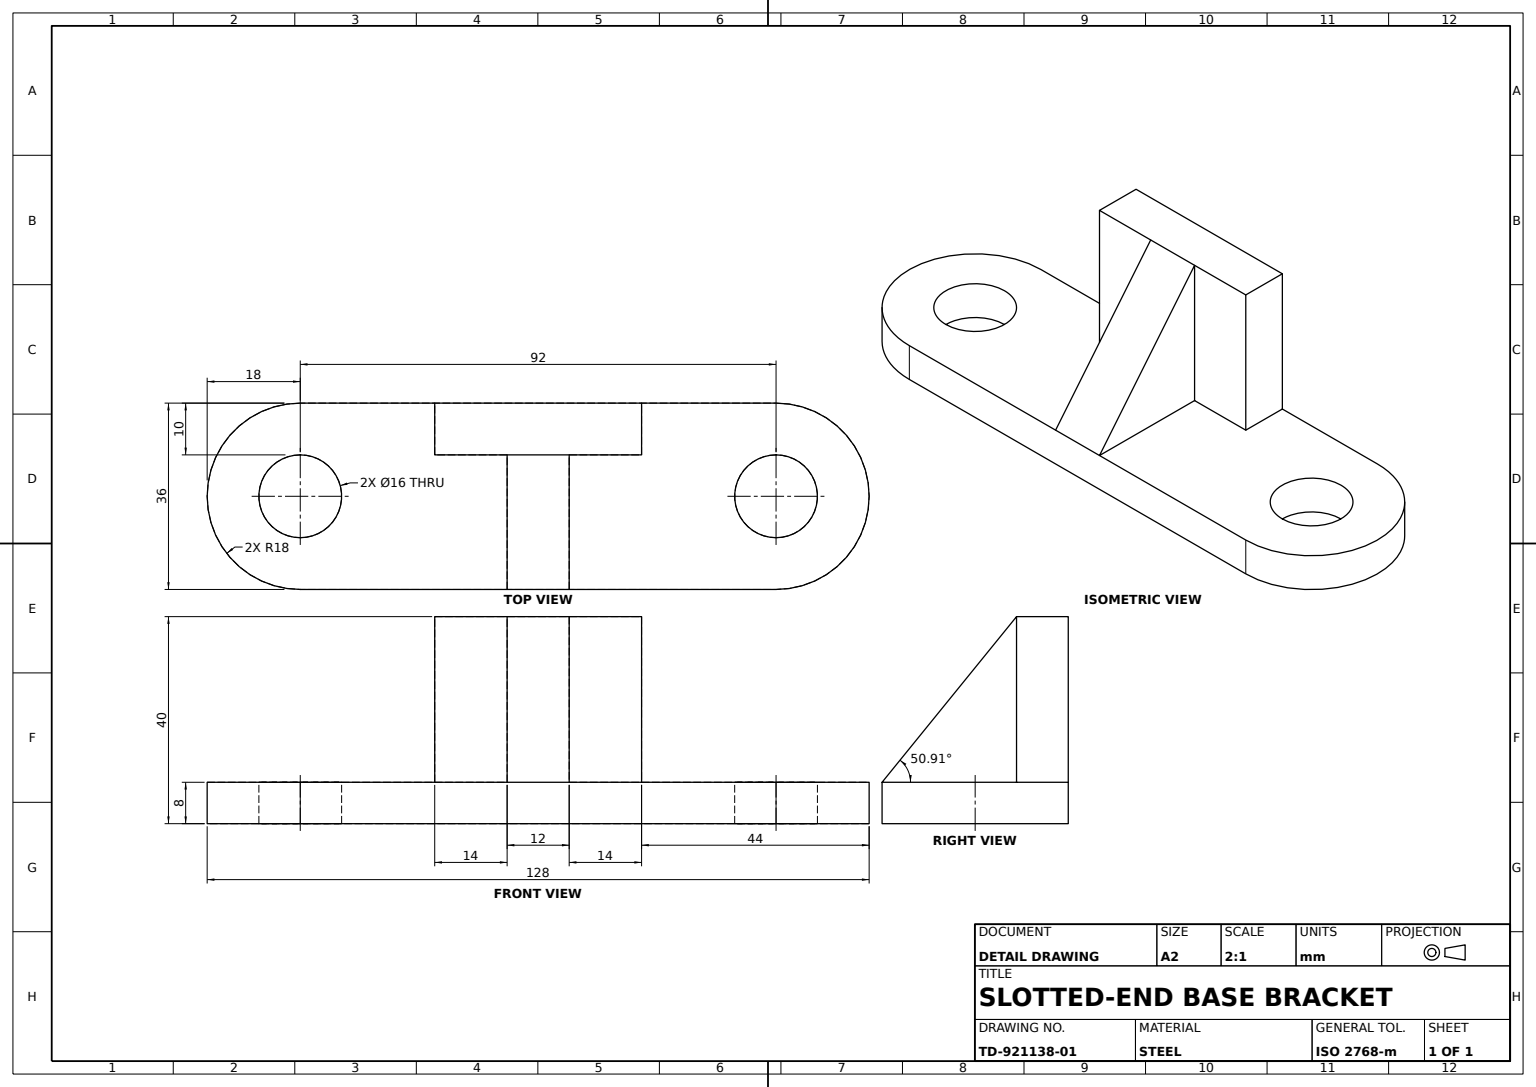
SolidWorks part; units mm, degrees
material "Plain Carbon Steel"
ref_plane "Front Plane" through (0, 0, 0) normal (0, 0, 1) x (1, 0, 0)
ref_plane "Top Plane" through (0, 0, 0) normal (0, 1, 0) x (1, 0, 0)
ref_plane "Right Plane" through (0, 0, 0) normal (1, 0, 0) x (0, 0, -1)
sketch "Base Plate Sketch" plane through (0, 0, 0) normal (0, 1, 0) x (1, 0, 0)
  line L0 (-46, 0) -> (46, 0) construction
  line L2 (-46, 18) -> (46, 18)
  line L3 (-46, -18) -> (46, -18)
  arc A0 (-46, 18) -> (-46, -18) centre (-46, 0) ccw
  arc A1 (46, -18) -> (46, 18) centre (46, 0) ccw
  point P5 (0, 0)
  dimension "D1" = 18
  dimension "D2" = 92
extrude "Base Plate" add sketch "Base Plate Sketch" along normal blind 8
sketch "Mounting Holes Sketch" plane through (0, 8, 0) normal (0, 1, 0) x (1, 0, 0)
  circle A0 centre (-46, 0) radius 8
  circle A1 centre (46, 0) radius 8
  dimension "D1" = 16
extrude "Mounting Holes 2x" cut sketch "Mounting Holes Sketch" against normal blind 8
sketch "Upright Sketch" plane through (0, 8, 0) normal (0, 1, 0) x (1, 0, 0)
  line L0 (0, 18) -> (-20, 18)
  line L1 (46, 18) -> (-46, 18) construction
  line L2 (-20, 18) -> (-20, 8)
  line L3 (-20, 8) -> (20, 8)
  line L4 (20, 8) -> (20, 18)
  line L5 (20, 18) -> (0, 18)
  dimension "D1" = 26
  dimension "D2" = 10
extrude "Upright" add sketch "Upright Sketch" along normal blind 32
sketch "Support Rib Sketch" plane through (0, 0, 0) normal (1, 0, 0) x (0, 0, -1)
  line L0 (8, 40) -> (-18, 8)
rib "Support Rib" sketch "Support Rib Sketch" sketch "Support Rib Sketch" thickness 12 extrusion direction parallel to sketch draft on no parameters "D1"=12
